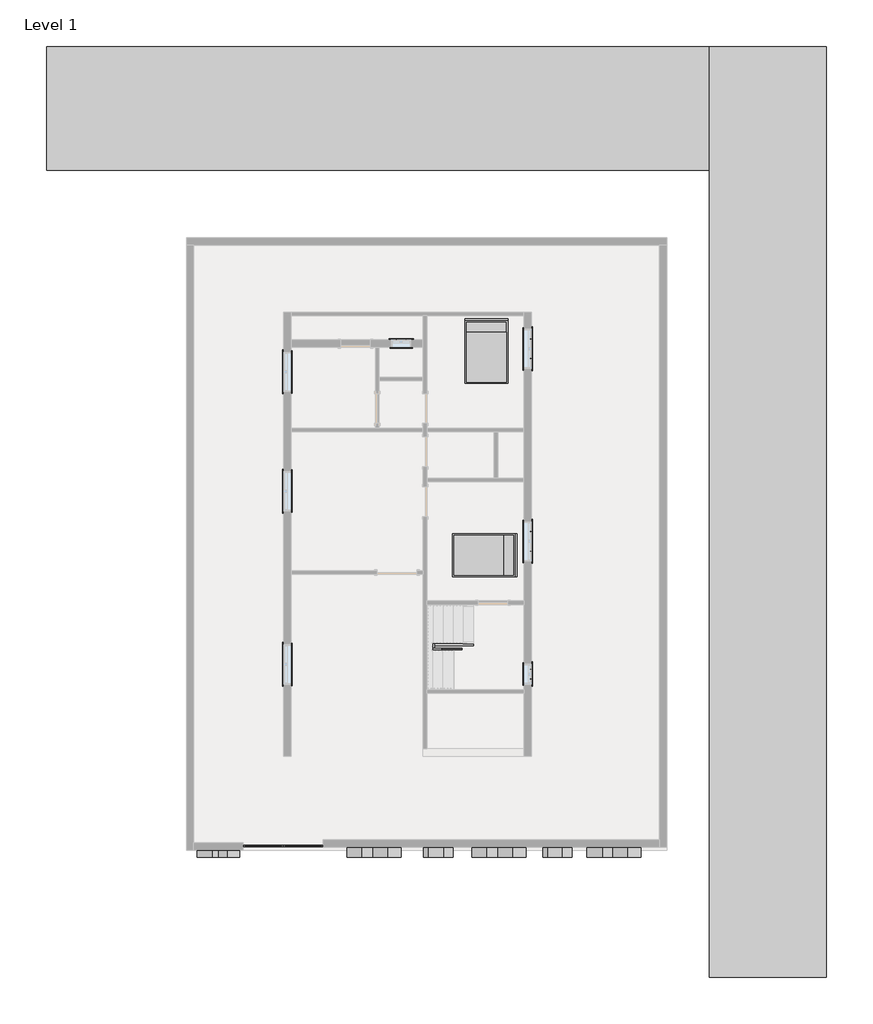
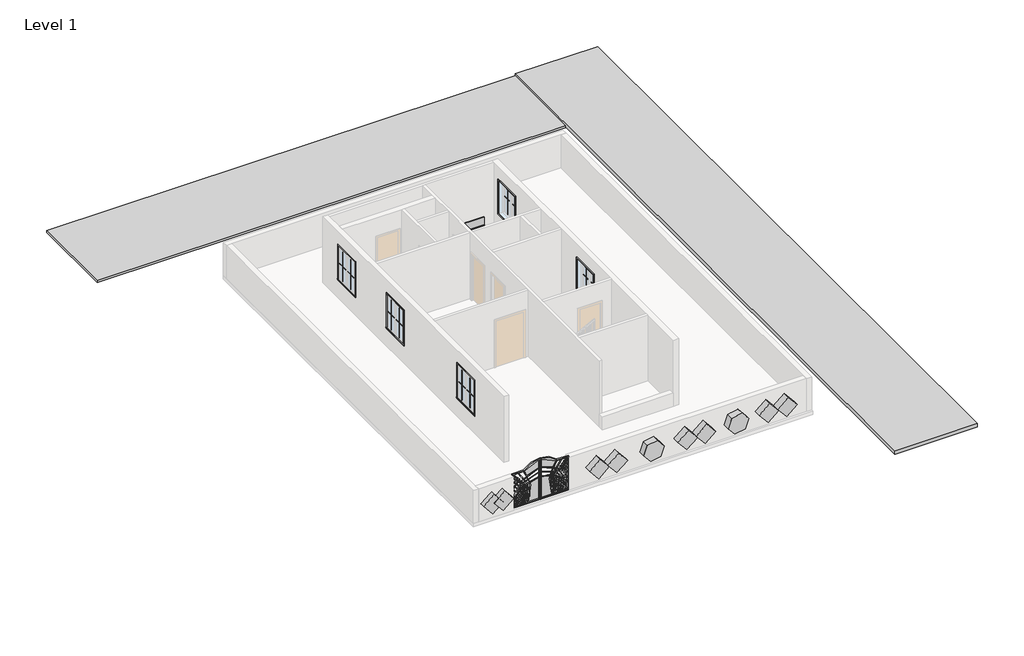
# One storey, part 7 of 7: 35 proxies, 5 members, 2 furniture elements.
"""IFC4 building model written with IfcOpenShell, lengths in millimetres."""

from ifc_helpers import new_model, si_unit, frame, origin, place, context, project, spatial, polyline, outline, extrude, transform, mapped, element, save
from components import generic_models_1_generic_models_1_1d0d8944, generic_models_2_generic_models_2_4ba01f5b, muntin_pattern_2x2_muntin_pattern_2x2_6dad3731, muntin_pattern_2x2_muntin_pattern_2x2_a30a3345, muntin_pattern_2x2_muntin_pattern_2x2_53152e2c, muntin_pattern_2x2_muntin_pattern_2x2_e8f3e573, trim_window_exterior_flat_with_sill_92b9b949, trim_window_exterior_flat_with_sill_a665a915, trim_window_interior_flat_picture_frame_3bb882cf, trim_window_interior_flat_picture_frame_d485c387, gate_7956_gate_7956_6bc30956, bed_17739_bed_17739_15c61121

model = new_model("IFC4")

# Units and contexts
model_context = context("Model", 3, world=origin())
ifc_project = project(units=[si_unit("LENGTHUNIT", "METRE", prefix="MILLI")], contexts=[model_context])

# Site, building, storey
site = spatial("IfcSite", under=ifc_project)
building = spatial("IfcBuilding", under=site)
storey = spatial("IfcBuildingStorey", under=building, Name="Level 1", Elevation=0.0)

# Proxies
placement = place(None, origin())
generic_models_1_generic_models_1_shape = generic_models_1_generic_models_1_1d0d8944(model_context)
element("IfcBuildingElementProxy", 1, Name="Generic Models 1 : Generic Models 1", ObjectType="Generic Models 1 : Generic Models 1", at=placement, inside=storey, context=model_context, shape_type="MappedRepresentation", body=[
    mapped(generic_models_1_generic_models_1_shape, transform((0.0, 0.0, 0.0), x_axis=(1.0, 0.0, 0.0), y_axis=(0.0, 1.0, 0.0), z_axis=(0.0, 0.0, 1.0))),
])
generic_models_2_generic_models_2_shape = generic_models_2_generic_models_2_4ba01f5b(model_context)
element("IfcBuildingElementProxy", 2, Name="Generic Models 2 : Generic Models 2", ObjectType="Generic Models 2 : Generic Models 2", at=placement, inside=storey, context=model_context, shape_type="MappedRepresentation", body=[
    mapped(generic_models_2_generic_models_2_shape, transform((0.0, 0.0, 0.0), x_axis=(1.0, 0.0, 0.0), y_axis=(0.0, 1.0, 0.0), z_axis=(0.0, 0.0, 1.0))),
])
muntin_pattern_2x2_muntin_pattern_2x2_shape = muntin_pattern_2x2_muntin_pattern_2x2_6dad3731(model_context)
element("IfcBuildingElementProxy", 3, Name="Muntin Pattern_2x2 : Muntin Pattern_2x2", ObjectType="Muntin Pattern_2x2 : Muntin Pattern_2x2", at=placement, inside=storey, context=model_context, shape_type="MappedRepresentation", body=[
    mapped(muntin_pattern_2x2_muntin_pattern_2x2_shape, transform((1279.525, 8669.3375, 984.25), x_axis=(0.0, 1.0, 0.0), y_axis=(-1.0, 0.0, 0.0), z_axis=(0.0, 0.0, 1.0))),
])
element("IfcBuildingElementProxy", 4, Name="Muntin Pattern_2x2 : Muntin Pattern_2x2", ObjectType="Muntin Pattern_2x2 : Muntin Pattern_2x2", at=placement, inside=storey, context=model_context, shape_type="MappedRepresentation", body=[
    mapped(muntin_pattern_2x2_muntin_pattern_2x2_shape, transform((1279.525, 3341.6875, 984.25), x_axis=(0.0, 1.0, 0.0), y_axis=(-1.0, 0.0, 0.0), z_axis=(0.0, 0.0, 1.0))),
])
element("IfcBuildingElementProxy", 5, Name="Muntin Pattern_2x2 : Muntin Pattern_2x2", ObjectType="Muntin Pattern_2x2 : Muntin Pattern_2x2", at=placement, inside=storey, context=model_context, shape_type="MappedRepresentation", body=[
    mapped(muntin_pattern_2x2_muntin_pattern_2x2_shape, transform((8880.475, 7732.7125, 984.25), x_axis=(0.0, -1.0, 0.0), y_axis=(1.0, 0.0, 0.0), z_axis=(0.0, 0.0, 1.0))),
])
element("IfcBuildingElementProxy", 6, Name="Muntin Pattern_2x2 : Muntin Pattern_2x2", ObjectType="Muntin Pattern_2x2 : Muntin Pattern_2x2", at=placement, inside=storey, context=model_context, shape_type="MappedRepresentation", body=[
    mapped(muntin_pattern_2x2_muntin_pattern_2x2_shape, transform((8880.475, 13657.2625, 984.25), x_axis=(0.0, -1.0, 0.0), y_axis=(1.0, 0.0, 0.0), z_axis=(0.0, 0.0, 1.0))),
])
element("IfcBuildingElementProxy", 7, Name="Muntin Pattern_2x2 : Muntin Pattern_2x2", ObjectType="Muntin Pattern_2x2 : Muntin Pattern_2x2", at=placement, inside=storey, context=model_context, shape_type="MappedRepresentation", body=[
    mapped(muntin_pattern_2x2_muntin_pattern_2x2_shape, transform((1279.525, 12339.6375, 984.25), x_axis=(0.0, 1.0, 0.0), y_axis=(-1.0, 0.0, 0.0), z_axis=(0.0, 0.0, 1.0))),
])
muntin_pattern_2x2_muntin_pattern_2x2_2_shape = muntin_pattern_2x2_muntin_pattern_2x2_a30a3345(model_context)
element("IfcBuildingElementProxy", 8, Name="Muntin Pattern_2x2 : Muntin Pattern_2x2", ObjectType="Muntin Pattern_2x2 : Muntin Pattern_2x2", at=placement, inside=storey, context=model_context, shape_type="MappedRepresentation", body=[
    mapped(muntin_pattern_2x2_muntin_pattern_2x2_2_shape, transform((1279.525, 9275.7625, 984.25), x_axis=(0.0, -1.0, 0.0), y_axis=(1.0, 0.0, 0.0), z_axis=(0.0, 0.0, 1.0))),
])
element("IfcBuildingElementProxy", 9, Name="Muntin Pattern_2x2 : Muntin Pattern_2x2", ObjectType="Muntin Pattern_2x2 : Muntin Pattern_2x2", at=placement, inside=storey, context=model_context, shape_type="MappedRepresentation", body=[
    mapped(muntin_pattern_2x2_muntin_pattern_2x2_2_shape, transform((1279.525, 3948.1125, 984.25), x_axis=(0.0, -1.0, 0.0), y_axis=(1.0, 0.0, 0.0), z_axis=(0.0, 0.0, 1.0))),
])
element("IfcBuildingElementProxy", 10, Name="Muntin Pattern_2x2 : Muntin Pattern_2x2", ObjectType="Muntin Pattern_2x2 : Muntin Pattern_2x2", at=placement, inside=storey, context=model_context, shape_type="MappedRepresentation", body=[
    mapped(muntin_pattern_2x2_muntin_pattern_2x2_2_shape, transform((8880.475, 7126.2875, 984.25), x_axis=(0.0, 1.0, 0.0), y_axis=(-1.0, 0.0, 0.0), z_axis=(0.0, 0.0, 1.0))),
])
element("IfcBuildingElementProxy", 11, Name="Muntin Pattern_2x2 : Muntin Pattern_2x2", ObjectType="Muntin Pattern_2x2 : Muntin Pattern_2x2", at=placement, inside=storey, context=model_context, shape_type="MappedRepresentation", body=[
    mapped(muntin_pattern_2x2_muntin_pattern_2x2_2_shape, transform((8880.475, 13050.8375, 984.25), x_axis=(0.0, 1.0, 0.0), y_axis=(-1.0, 0.0, 0.0), z_axis=(0.0, 0.0, 1.0))),
])
element("IfcBuildingElementProxy", 12, Name="Muntin Pattern_2x2 : Muntin Pattern_2x2", ObjectType="Muntin Pattern_2x2 : Muntin Pattern_2x2", at=placement, inside=storey, context=model_context, shape_type="MappedRepresentation", body=[
    mapped(muntin_pattern_2x2_muntin_pattern_2x2_2_shape, transform((1279.525, 12946.0625, 984.25), x_axis=(0.0, -1.0, 0.0), y_axis=(1.0, 0.0, 0.0), z_axis=(0.0, 0.0, 1.0))),
])
muntin_pattern_2x2_muntin_pattern_2x2_3_shape = muntin_pattern_2x2_muntin_pattern_2x2_53152e2c(model_context)
element("IfcBuildingElementProxy", 13, Name="Muntin Pattern_2x2 : Muntin Pattern_2x2", ObjectType="Muntin Pattern_2x2 : Muntin Pattern_2x2", at=placement, inside=storey, context=model_context, shape_type="MappedRepresentation", body=[
    mapped(muntin_pattern_2x2_muntin_pattern_2x2_3_shape, transform((4732.3375, 13617.575, 984.25), x_axis=(1.0, 0.0, 0.0), y_axis=(0.0, 1.0, 0.0), z_axis=(0.0, 0.0, 1.0))),
])
element("IfcBuildingElementProxy", 14, Name="Muntin Pattern_2x2 : Muntin Pattern_2x2", ObjectType="Muntin Pattern_2x2 : Muntin Pattern_2x2", at=placement, inside=storey, context=model_context, shape_type="MappedRepresentation", body=[
    mapped(muntin_pattern_2x2_muntin_pattern_2x2_3_shape, transform((8880.475, 3497.2625, 984.25), x_axis=(0.0, -1.0, 0.0), y_axis=(1.0, 0.0, 0.0), z_axis=(0.0, 0.0, 1.0))),
])
element("IfcBuildingElementProxy", 15, Name="Muntin Pattern_2x2 : Muntin Pattern_2x2", ObjectType="Muntin Pattern_2x2 : Muntin Pattern_2x2", at=placement, inside=storey, context=model_context, shape_type="MappedRepresentation", body=[
    mapped(muntin_pattern_2x2_muntin_pattern_2x2_3_shape, transform((4732.3375, 13617.575, 984.25), x_axis=(1.0, 0.0, 0.0), y_axis=(0.0, 1.0, 0.0), z_axis=(0.0, 0.0, 1.0))),
])
muntin_pattern_2x2_muntin_pattern_2x2_4_shape = muntin_pattern_2x2_muntin_pattern_2x2_e8f3e573(model_context)
element("IfcBuildingElementProxy", 16, Name="Muntin Pattern_2x2 : Muntin Pattern_2x2", ObjectType="Muntin Pattern_2x2 : Muntin Pattern_2x2", at=placement, inside=storey, context=model_context, shape_type="MappedRepresentation", body=[
    mapped(muntin_pattern_2x2_muntin_pattern_2x2_4_shape, transform((5033.9625, 13617.575, 984.25), x_axis=(-1.0, 0.0, 0.0), y_axis=(0.0, -1.0, 0.0), z_axis=(0.0, 0.0, 1.0))),
])
element("IfcBuildingElementProxy", 17, Name="Muntin Pattern_2x2 : Muntin Pattern_2x2", ObjectType="Muntin Pattern_2x2 : Muntin Pattern_2x2", at=placement, inside=storey, context=model_context, shape_type="MappedRepresentation", body=[
    mapped(muntin_pattern_2x2_muntin_pattern_2x2_4_shape, transform((8880.475, 3195.6375, 984.25), x_axis=(0.0, 1.0, 0.0), y_axis=(-1.0, 0.0, 0.0), z_axis=(0.0, 0.0, 1.0))),
])
element("IfcBuildingElementProxy", 18, Name="Muntin Pattern_2x2 : Muntin Pattern_2x2", ObjectType="Muntin Pattern_2x2 : Muntin Pattern_2x2", at=placement, inside=storey, context=model_context, shape_type="MappedRepresentation", body=[
    mapped(muntin_pattern_2x2_muntin_pattern_2x2_4_shape, transform((5033.9625, 13617.575, 984.25), x_axis=(-1.0, 0.0, 0.0), y_axis=(0.0, -1.0, 0.0), z_axis=(0.0, 0.0, 1.0))),
])
trim_window_exterior_flat_with_sill_shape = trim_window_exterior_flat_with_sill_92b9b949(model_context)
element("IfcBuildingElementProxy", 19, Name="Trim-Window-Exterior-Flat : with Sill", ObjectType="Trim-Window-Exterior-Flat : with Sill", at=placement, inside=storey, context=model_context, shape_type="MappedRepresentation", body=[
    mapped(trim_window_exterior_flat_with_sill_shape, transform((1270.0, 8972.55, 2438.4), x_axis=(0.0, -1.0, 0.0), y_axis=(0.0, 0.0, 1.0), z_axis=(-1.0, 0.0, 0.0))),
])
element("IfcBuildingElementProxy", 20, Name="Trim-Window-Exterior-Flat : with Sill", ObjectType="Trim-Window-Exterior-Flat : with Sill", at=placement, inside=storey, context=model_context, shape_type="MappedRepresentation", body=[
    mapped(trim_window_exterior_flat_with_sill_shape, transform((1270.0, 3644.9, 2438.4), x_axis=(0.0, -1.0, 0.0), y_axis=(0.0, 0.0, 1.0), z_axis=(-1.0, 0.0, 0.0))),
])
element("IfcBuildingElementProxy", 21, Name="Trim-Window-Exterior-Flat : with Sill", ObjectType="Trim-Window-Exterior-Flat : with Sill", at=placement, inside=storey, context=model_context, shape_type="MappedRepresentation", body=[
    mapped(trim_window_exterior_flat_with_sill_shape, transform((8890.0, 7429.5, 2438.4), x_axis=(0.0, 1.0, 0.0), y_axis=(0.0, 0.0, 1.0), z_axis=(1.0, 0.0, 0.0))),
])
element("IfcBuildingElementProxy", 22, Name="Trim-Window-Exterior-Flat : with Sill", ObjectType="Trim-Window-Exterior-Flat : with Sill", at=placement, inside=storey, context=model_context, shape_type="MappedRepresentation", body=[
    mapped(trim_window_exterior_flat_with_sill_shape, transform((8890.0, 13354.05, 2438.4), x_axis=(0.0, 1.0, 0.0), y_axis=(0.0, 0.0, 1.0), z_axis=(1.0, 0.0, 0.0))),
])
element("IfcBuildingElementProxy", 23, Name="Trim-Window-Exterior-Flat : with Sill", ObjectType="Trim-Window-Exterior-Flat : with Sill", at=placement, inside=storey, context=model_context, shape_type="MappedRepresentation", body=[
    mapped(trim_window_exterior_flat_with_sill_shape, transform((1270.0, 12642.85, 2438.4), x_axis=(0.0, -1.0, 0.0), y_axis=(0.0, 0.0, 1.0), z_axis=(-1.0, 0.0, 0.0))),
])
trim_window_exterior_flat_with_sill_2_shape = trim_window_exterior_flat_with_sill_a665a915(model_context)
element("IfcBuildingElementProxy", 24, Name="Trim-Window-Exterior-Flat : with Sill", ObjectType="Trim-Window-Exterior-Flat : with Sill", at=placement, inside=storey, context=model_context, shape_type="MappedRepresentation", body=[
    mapped(trim_window_exterior_flat_with_sill_2_shape, transform((4883.15, 13627.1, 1828.8), x_axis=(-1.0, 0.0, 0.0), y_axis=(0.0, 0.0, 1.0), z_axis=(0.0, 1.0, 0.0))),
])
element("IfcBuildingElementProxy", 25, Name="Trim-Window-Exterior-Flat : with Sill", ObjectType="Trim-Window-Exterior-Flat : with Sill", at=placement, inside=storey, context=model_context, shape_type="MappedRepresentation", body=[
    mapped(trim_window_exterior_flat_with_sill_2_shape, transform((8890.0, 3346.45, 1828.8), x_axis=(0.0, 1.0, 0.0), y_axis=(0.0, 0.0, 1.0), z_axis=(1.0, 0.0, 0.0))),
])
element("IfcBuildingElementProxy", 26, Name="Trim-Window-Exterior-Flat : with Sill", ObjectType="Trim-Window-Exterior-Flat : with Sill", at=placement, inside=storey, context=model_context, shape_type="MappedRepresentation", body=[
    mapped(trim_window_exterior_flat_with_sill_2_shape, transform((4883.15, 13627.1, 1828.8), x_axis=(-1.0, 0.0, 0.0), y_axis=(0.0, 0.0, 1.0), z_axis=(0.0, 1.0, 0.0))),
])
trim_window_interior_flat_picture_frame_shape = trim_window_interior_flat_picture_frame_3bb882cf(model_context)
element("IfcBuildingElementProxy", 27, Name="Trim-Window-Interior-Flat : Picture Frame", ObjectType="Trim-Window-Interior-Flat : Picture Frame", at=placement, inside=storey, context=model_context, shape_type="MappedRepresentation", body=[
    mapped(trim_window_interior_flat_picture_frame_shape, transform((1498.6, 8972.55, 2438.4), x_axis=(0.0, 1.0, 0.0), y_axis=(0.0, 0.0, 1.0), z_axis=(1.0, 0.0, 0.0))),
])
element("IfcBuildingElementProxy", 28, Name="Trim-Window-Interior-Flat : Picture Frame", ObjectType="Trim-Window-Interior-Flat : Picture Frame", at=placement, inside=storey, context=model_context, shape_type="MappedRepresentation", body=[
    mapped(trim_window_interior_flat_picture_frame_shape, transform((1498.6, 3644.9, 2438.4), x_axis=(0.0, 1.0, 0.0), y_axis=(0.0, 0.0, 1.0), z_axis=(1.0, 0.0, 0.0))),
])
element("IfcBuildingElementProxy", 29, Name="Trim-Window-Interior-Flat : Picture Frame", ObjectType="Trim-Window-Interior-Flat : Picture Frame", at=placement, inside=storey, context=model_context, shape_type="MappedRepresentation", body=[
    mapped(trim_window_interior_flat_picture_frame_shape, transform((8661.4, 7429.5, 2438.4), x_axis=(0.0, -1.0, 0.0), y_axis=(0.0, 0.0, 1.0), z_axis=(-1.0, 0.0, 0.0))),
])
element("IfcBuildingElementProxy", 30, Name="Trim-Window-Interior-Flat : Picture Frame", ObjectType="Trim-Window-Interior-Flat : Picture Frame", at=placement, inside=storey, context=model_context, shape_type="MappedRepresentation", body=[
    mapped(trim_window_interior_flat_picture_frame_shape, transform((8661.4, 13354.05, 2438.4), x_axis=(0.0, -1.0, 0.0), y_axis=(0.0, 0.0, 1.0), z_axis=(-1.0, 0.0, 0.0))),
])
element("IfcBuildingElementProxy", 31, Name="Trim-Window-Interior-Flat : Picture Frame", ObjectType="Trim-Window-Interior-Flat : Picture Frame", at=placement, inside=storey, context=model_context, shape_type="MappedRepresentation", body=[
    mapped(trim_window_interior_flat_picture_frame_shape, transform((1498.6, 12642.85, 2438.4), x_axis=(0.0, 1.0, 0.0), y_axis=(0.0, 0.0, 1.0), z_axis=(1.0, 0.0, 0.0))),
])
trim_window_interior_flat_picture_frame_2_shape = trim_window_interior_flat_picture_frame_d485c387(model_context)
element("IfcBuildingElementProxy", 32, Name="Trim-Window-Interior-Flat : Picture Frame", ObjectType="Trim-Window-Interior-Flat : Picture Frame", at=placement, inside=storey, context=model_context, shape_type="MappedRepresentation", body=[
    mapped(trim_window_interior_flat_picture_frame_2_shape, transform((4883.15, 13398.5, 1828.8), x_axis=(1.0, 0.0, 0.0), y_axis=(0.0, 0.0, 1.0), z_axis=(0.0, -1.0, 0.0))),
])
element("IfcBuildingElementProxy", 33, Name="Trim-Window-Interior-Flat : Picture Frame", ObjectType="Trim-Window-Interior-Flat : Picture Frame", at=placement, inside=storey, context=model_context, shape_type="MappedRepresentation", body=[
    mapped(trim_window_interior_flat_picture_frame_2_shape, transform((8661.4, 3346.45, 1828.8), x_axis=(0.0, -1.0, 0.0), y_axis=(0.0, 0.0, 1.0), z_axis=(-1.0, 0.0, 0.0))),
])
element("IfcBuildingElementProxy", 34, Name="Trim-Window-Interior-Flat : Picture Frame", ObjectType="Trim-Window-Interior-Flat : Picture Frame", at=placement, inside=storey, context=model_context, shape_type="MappedRepresentation", body=[
    mapped(trim_window_interior_flat_picture_frame_2_shape, transform((4883.15, 13398.5, 1828.8), x_axis=(1.0, 0.0, 0.0), y_axis=(0.0, 0.0, 1.0), z_axis=(0.0, -1.0, 0.0))),
])
gate_7956_gate_7956_shape = gate_7956_gate_7956_6bc30956(model_context)
element("IfcBuildingElementProxy", 35, Name="gate_7956 : gate_7956", ObjectType="gate_7956 : gate_7956", at=placement, inside=storey, context=model_context, shape_type="MappedRepresentation", body=[
    mapped(gate_7956_gate_7956_shape, transform((1255.0106944, -1918.0474619, 0.0), x_axis=(1.0, 0.0, 0.0), y_axis=(0.0, 1.0, 0.0), z_axis=(0.0, 0.0, 1.0))),
])

# Furniture
bed_17739_bed_17739_shape = bed_17739_bed_17739_15c61121(model_context)
element("IfcFurniture", 36, ObjectType="Bed_17739 : Bed_17739", at=placement, inside=storey, context=model_context, shape_type="MappedRepresentation", body=[
    mapped(bed_17739_bed_17739_shape, transform((7429.5, 7004.05, 0.0), x_axis=(0.0, -1.0, 0.0), y_axis=(1.0, 0.0, 0.0), z_axis=(0.0, 0.0, 1.0))),
])
element("IfcFurniture", 37, ObjectType="Bed_17739 : Bed_17739", at=placement, inside=storey, context=model_context, shape_type="MappedRepresentation", body=[
    mapped(bed_17739_bed_17739_shape, transform((7505.7, 13258.8, 0.0), x_axis=(1.0, 0.0, 0.0), y_axis=(0.0, 1.0, 0.0), z_axis=(0.0, 0.0, 1.0))),
])

# Members
element("IfcMember", 38, ObjectType="Stringer - 2\" Width", at=placement, inside=storey, context=model_context, shape_type="SweptSolid", body=[
    extrude(outline(polyline([(0.0, 7105.1820958), (198.2547253, 7105.1820958), (856.5684612, 5911.3820958), (508.4966856, 5911.3820958), (0.0, 6833.5007001), (0.0, 7105.1820958)])), frame((0.0, 4223.8882626, 0.0), z_axis=(0.0, 1.0, 0.0), x_axis=(0.0, 0.0, 1.0)), (0.0, 0.0, 1.0), 50.8),
])
element("IfcMember", 39, ObjectType="Stringer - 2\" Width", at=placement, inside=storey, context=model_context, shape_type="SweptSolid", body=[
    extrude(outline(polyline([(5860.5820958, 4274.6882626), (5911.3820958, 4274.6882626), (5911.3820958, 4147.6882626), (5860.5820958, 4147.6882626), (5860.5820958, 4274.6882626)])), frame((0.0, 0.0, 618.0666667), z_axis=(0.0, 0.0, 1.0), x_axis=(1.0, 0.0, 0.0)), (0.0, 0.0, 1.0), 304.8),
])
element("IfcMember", 40, ObjectType="Stringer - 2\" Width", at=placement, inside=storey, context=model_context, shape_type="SweptSolid", body=[
    extrude(outline(polyline([(1053.9151449, 5860.5820958), (705.8433694, 5860.5820958), (1392.1704557, 7105.1820958), (1740.2422312, 7105.1820958), (1053.9151449, 5860.5820958)])), frame((0.0, 4096.8882626, 0.0), z_axis=(0.0, 1.0, 0.0), x_axis=(0.0, 0.0, 1.0)), (0.0, 0.0, 1.0), 50.8),
])
element("IfcMember", 41, ObjectType="Stringer - 2\" Width", at=placement, inside=storey, context=model_context, shape_type="SweptSolid", body=[
    extrude(outline(polyline([(0.0, 7105.1820958), (198.2547253, 7105.1820958), (922.8666667, 5791.155533), (922.8666667, 5676.9), (637.8004086, 5676.9), (0.0, 6833.5007001), (0.0, 7105.1820958)])), frame((0.0, 5486.4, 0.0), z_axis=(0.0, 1.0, 0.0), x_axis=(0.0, 0.0, 1.0)), (0.0, 0.0, 1.0), 50.8),
])
element("IfcMember", 42, ObjectType="Stringer - 2\" Width", at=placement, inside=storey, context=model_context, shape_type="SweptSolid", body=[
    extrude(outline(polyline([(5626.1, 5537.2), (5676.9, 5537.2), (5676.9, 2870.2), (5626.1, 2870.2), (5626.1, 5537.2)])), frame((0.0, 0.0, 618.0666667), z_axis=(0.0, 0.0, 1.0), x_axis=(1.0, 0.0, 0.0)), (0.0, 0.0, 1.0), 304.8),
])

save(model, "model.ifc")

# Revit data of these elements
# Type "Muntin Pattern_2x2 : Muntin Pattern_2x2"
#   Width [instance default] = 4' - 0"
#   Thickness = 0' - 0 1/2"
#   Height [instance default] = 4' - 0"
#   Distance = 0' - 0 3/4"
#   Interior Material [instance default] = none
#   Exterior Material [instance default] = none
#   Default Elevation = 0
# Type "Trim-Window-Exterior-Flat : with Sill"
#   Trim Width = 0' - 2 1/4"
#   Trim Thickness_Picture Frame = 0' - 1 1/4"
#   Trim Thickness_with Sill = 0' - 0 3/4"
#   Sill Thickness = 0' - 1 1/4"
#   Opening Width [instance default] = 2' - 0"
#   Opening Height [instance default] = 3' - 0"
#   Default Elevation = 4' - 0"
#   Sill = yes
#   Picture Frame = no
#   Trim Material [instance default] = none
# Type "Trim-Window-Interior-Flat : Picture Frame"
#   Trim Thickness_Picture Frame = 0' - 1 1/4"
#   Trim Width = 0' - 2 1/4"
#   Trim Thickness_with Sill = 0' - 0 3/4"
#   Sill Thickness = 0' - 1 1/4"
#   Opening Width [instance default] = 2' - 0"
#   Opening Height [instance default] = 3' - 0"
#   Default Elevation = 4' - 0"
#   Sill = no
#   Picture Frame = yes
#   Trim Material [instance default] = none
# Type "gate_7956 : gate_7956"
#   m.s. sheet = none
#   2" x2" pipe = none
#   1"x1"pipe = none
#   Default Elevation = 0
# Type "Bed_17739 : Bed_17739"
#   Default Elevation = 0
# Element 1 (IfcBuildingElementProxy, "Generic Models 1 : Generic Models 1")
#   Phase Created = New Construction
# Element 2 (IfcBuildingElementProxy, "Generic Models 2 : Generic Models 2")
#   Phase Created = New Construction
#   Materials on its faces: "Cherry", "Clad - White"
# Elements 3, 4, 5, 6, 7, 8, 9, 10, 11, 12 (IfcBuildingElementProxy, "Muntin Pattern_2x2 : Muntin Pattern_2x2")
#   Width = 1' - 6 5/8"
#   Height = 4' - 6 1/2"
#   Interior Material = Wood - Stained
#   Exterior Material = Clad - White
#   Phase Created = New Construction
#   Materials on its faces: "Clad - White", "Wood - Stained"
# Elements 13, 14, 15, 16, 17, 18 (IfcBuildingElementProxy, "Muntin Pattern_2x2 : Muntin Pattern_2x2")
#   Width = 0' - 6 5/8"
#   Height = 2' - 6 1/2"
#   Interior Material = Wood - Stained
#   Exterior Material = Clad - White
#   Phase Created = New Construction
#   Materials on its faces: "Clad - White", "Wood - Stained"
# Elements 19, 20, 21, 22, 23 (IfcBuildingElementProxy, "Trim-Window-Exterior-Flat : with Sill")
#   Opening Width = 4' - 0"
#   Opening Height = 5' - 0"
#   Trim Material = Clad - White
#   Phase Created = New Construction
#   Materials on its faces: "Clad - White"
# Elements 24, 25, 26 (IfcBuildingElementProxy, "Trim-Window-Exterior-Flat : with Sill")
#   Opening Width = 2' - 0"
#   Opening Height = 3' - 0"
#   Trim Material = Clad - White
#   Phase Created = New Construction
#   Materials on its faces: "Clad - White"
# Elements 27, 28, 29, 30, 31 (IfcBuildingElementProxy, "Trim-Window-Interior-Flat : Picture Frame")
#   Opening Width = 4' - 0"
#   Opening Height = 5' - 0"
#   Trim Material = Wood - Stained
#   Phase Created = New Construction
#   Materials on its faces: "Wood - Stained"
# Elements 32, 33, 34 (IfcBuildingElementProxy, "Trim-Window-Interior-Flat : Picture Frame")
#   Opening Width = 2' - 0"
#   Opening Height = 3' - 0"
#   Trim Material = Wood - Stained
#   Phase Created = New Construction
#   Materials on its faces: "Wood - Stained"
# Element 35 (IfcBuildingElementProxy, "gate_7956 : gate_7956")
#   Phase Created = New Construction
#   Materials on its faces: "r1"
# Elements 36, 37 (IfcFurniture, "Bed_17739 : Bed_17739")
#   Phase Created = New Construction
#   Materials on its faces: "legs", "sheets", "bed frame", "Blanket"
# Elements 38, 39, 40, 41, 42 (IfcMember, "Stringer - 2\" Width")
#   Phase Created = New Construction
# Materials
#   "Cherry": class "Wood", colour RGB 226 177 128, transparency 0, Description = "Prunus Serotina", Cost = 0
#   "Clad - White": class "Wood", colour RGB 242 242 238, transparency 0, Cost = 0
#   "Wood - Stained": class "Wood", colour RGB 224 178 126, transparency 0, Cost = 0
#   "r1": class "Generic", colour RGB 120 120 120, transparency 0, Cost = 0
#   "legs": colour RGB 90 73 37, transparency 0, Cost = 0
#   "sheets": colour RGB 200 195 176, transparency 0, Cost = 0
#   "bed frame": colour RGB 90 73 37, transparency 0, Cost = 0
#   "Blanket": class "System", colour RGB 59 0 1, transparency 0, Cost = 0
